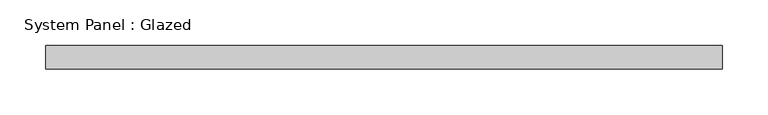
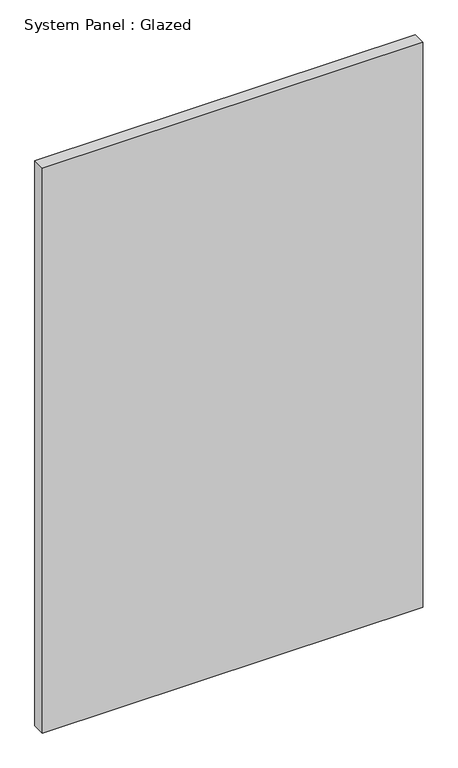
"""IFC4 building model written with IfcOpenShell, lengths in millimetres: plate geometry, System Panel : Glazed."""

from ifc_helpers import new_model, si_unit, origin, origin_with_axes, place, context, project, spatial, polyline, outline, extrude, source, transform, mapped, element, save


def system_panel_glazed_b1e6bfa8(model_context):
    return source(origin(), model_context, "Body", "SweptSolid", [
        extrude(outline(polyline([(368.3, 19.05), (-368.3, 19.05), (-368.3, 44.45), (368.3, 44.45), (368.3, 19.05)])), origin_with_axes(), (0.0, 0.0, 1.0), 1155.7),
    ])


if __name__ == "__main__":
    model = new_model("IFC4")
    model_context = context("Model", 3, world=origin())
    ifc_project = project(units=[si_unit("LENGTHUNIT", "METRE", prefix="MILLI")], contexts=[model_context])
    site = spatial("IfcSite", under=ifc_project)
    building = spatial("IfcBuilding", under=site)
    placement = place(None, origin())
    system_panel_glazed_shape = system_panel_glazed_b1e6bfa8(model_context)
    element("IfcPlate", 1, ObjectType="System Panel : Glazed", at=placement, inside=building, context=model_context, shape_type="MappedRepresentation", body=[
        mapped(system_panel_glazed_shape, transform((0.0, 0.0, 0.0), x_axis=(1.0, 0.0, 0.0), y_axis=(0.0, 1.0, 0.0), z_axis=(0.0, 0.0, 1.0))),
    ])
    save(model, "model.ifc")

# Revit data of these elements
# Type "System Panel : Glazed"
#   Construction Type Id = "GSP4R"
#   Analytic Construction = "1/8 in Pilkington single glazing"
#   Visual Light Transmittance = 0.9
#   Solar Heat Gain Coefficient = 0.86
#   Heat Transfer Coefficient (U) = 1.18115 BTU/(h·ft²·°F)
# Element 1 (IfcPlate, "System Panel : Glazed")
#   Materials on its faces: "Glass"
# Materials
#   "Glass": class "Glass", colour RGB 0 128 192, transparency 0.75, Description = "Soda Lime Glass", Cost = 0
